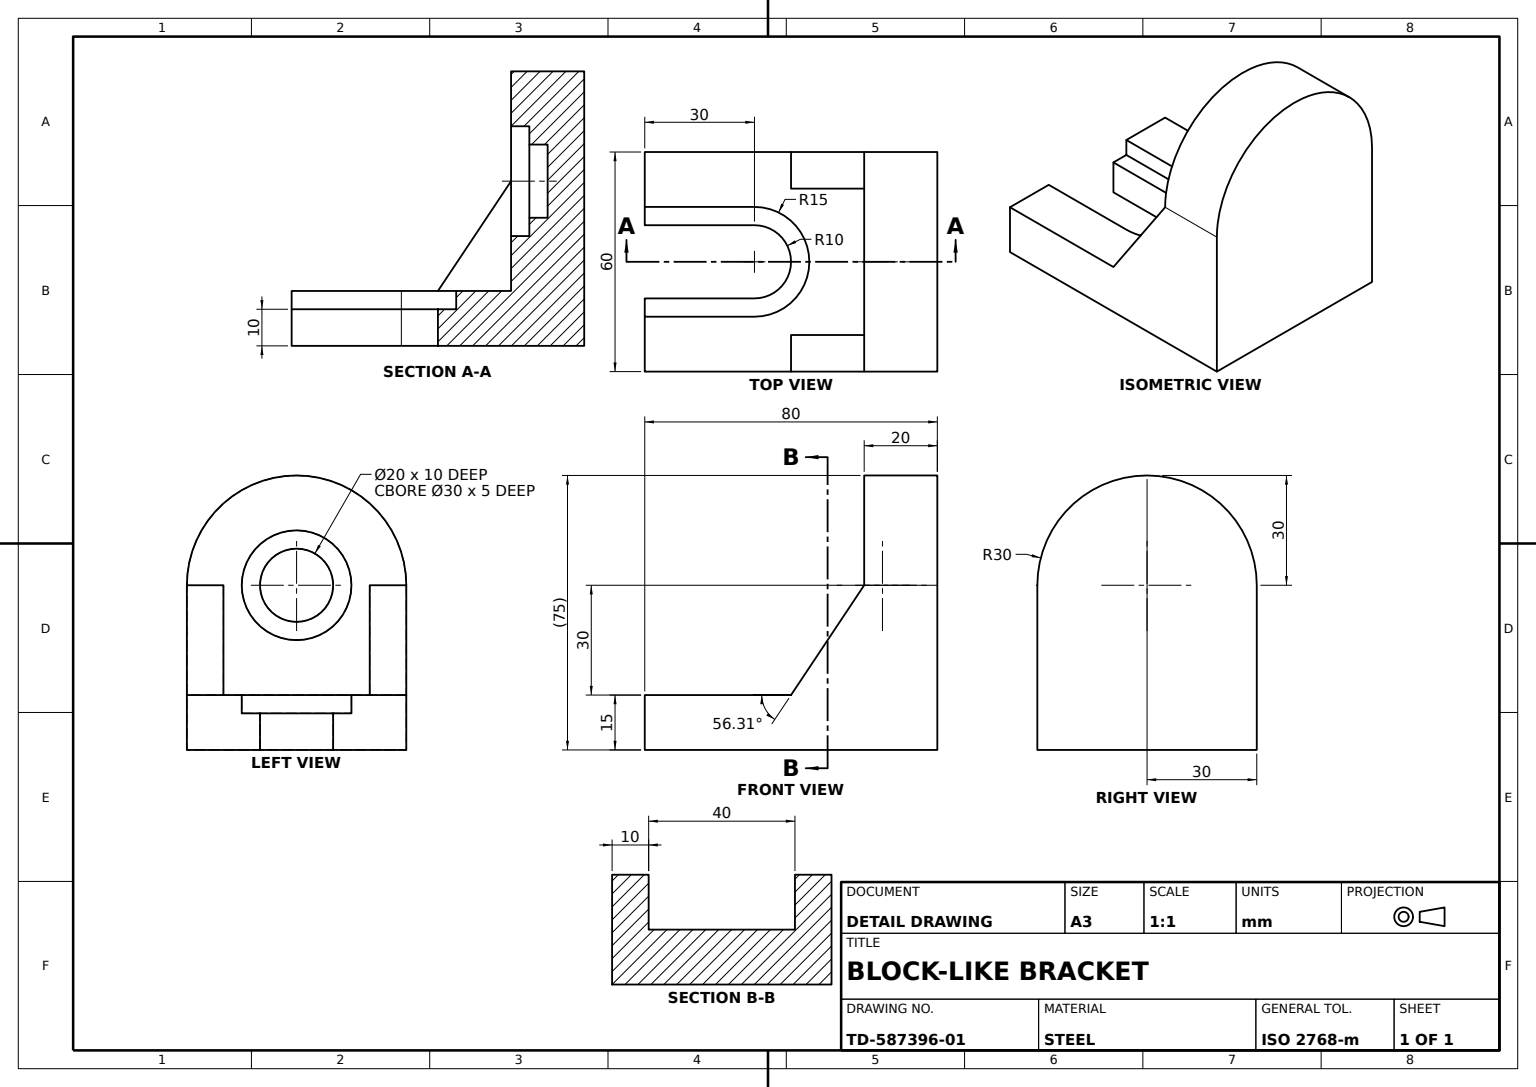
SolidWorks part; units mm, degrees
material "Plain Carbon Steel"
ref_plane "Front Plane" through (0, 0, 0) normal (0, 0, 1) x (1, 0, 0)
ref_plane "Top Plane" through (0, 0, 0) normal (0, 1, 0) x (1, 0, 0)
ref_plane "Right Plane" through (0, 0, 0) normal (1, 0, 0) x (0, 0, -1)
sketch "Base Plate Sketch" plane through (0, 0, 0) normal (0, 0, 1) x (1, 0, 0)
  line L0 (0, 0) -> (80, 0)
  line L1 (80, 0) -> (80, 60)
  line L2 (80, 60) -> (0, 60)
  line L3 (0, 60) -> (0, 0)
  dimension "D1" = 80
  dimension "D2" = 60
extrude "Base Plate" add sketch "Base Plate Sketch" along normal blind 15
sketch "Upright Block Sketch" plane through (80, 0, 0) normal (1, 0, 0) x (0, 0, -1)
  line L0 (-15, 60) -> (-45, 60)
  line L2 (-45, 0) -> (-15, 0)
  line L3 (-15, 0) -> (-15, 60) construction
  line L4 (-15, 0) -> (-15, 60)
  arc A0 (-45, 60) -> (-45, 0) centre (-45, 30) ccw
  dimension "D1" = 60
extrude "Upright Block" add sketch "Upright Block Sketch" against normal blind 20
sketch "Recess Ø30 Sketch" plane through (60, 0, 0) normal (-1, 0, 0) x (0, 0, 1)
  circle A0 centre (45, 30) radius 15
  dimension "D1" = 30
  dimension "D2" = 30
extrude "Recess Ø30" cut sketch "Recess Ø30 Sketch" against normal blind 5
sketch "Recess Ø20 Sketch" plane through (65, 0, 0) normal (-1, 0, 0) x (0, 0, 1)
  circle A0 centre (45, 30) radius 10
  dimension "D1" = 20
  dimension "D2" = 20
extrude "Recess Ø20" cut sketch "Recess Ø20 Sketch" against normal blind 5
sketch "Slot 30 Sketch" plane through (0, 0, 15) normal (0, 0, 1) x (1, 0, 0)
  line L0 (0, 45) -> (0, 15)
  line L1 (0, 60) -> (0, 0) construction
  line L2 (0, 45) -> (30, 45)
  line L4 (30, 15) -> (0, 15)
  line L5 (0, 0) -> (60, 0) construction
  arc A0 (30, 15) -> (30, 45) centre (30, 30) ccw
  dimension "D1" = 30
  dimension "D2" = 15
  dimension "D3" = 30
extrude "Slot 30" cut sketch "Slot 30 Sketch" against normal blind 5
sketch "Slot Step 20 Sketch" plane through (0, 0, 10) normal (0, 0, 1) x (1, 0, 0)
  line L0 (30, 45) -> (0, 45) construction
  line L1 (0, 45) -> (0, 15) construction
  line L2 (0, 40) -> (30, 40)
  line L4 (0, 20) -> (30, 20)
  line L5 (0, 40) -> (0, 20)
  arc A0 (30, 20) -> (30, 40) centre (30, 30) ccw
  dimension "D1" = 20
  dimension "D2" = 10
  dimension "D3" = 30
  dimension "D4" = 15
extrude "Slot Step 20" cut sketch "Slot Step 20 Sketch" against normal blind 10
sketch "Side Boss Sketch" plane through (0, 0, 0) normal (0, -1, 0) x (1, 0, 0)
  line L0 (60, 45) -> (40, 15)
  line L1 (0, 15) -> (60, 15) construction
  line L2 (60, 45) -> (80, 45) construction
  line L3 (60, 45) -> (60, 15)
  line L4 (60, 15) -> (40, 15)
  point P7 (70, 45)
  dimension "D1" = 30
extrude "Side Boss" add sketch "Side Boss Sketch" against normal blind 10
sketch "Rounded Boss Sketch" plane through (0, 60, 0) normal (0, 1, 0) x (1, 0, 0)
  line L0 (40, -15) -> (60, -15)
  line L1 (60, -15) -> (60, -45)
  line L2 (60, -45) -> (40, -15)
extrude "Rounded Boss" add sketch "Rounded Boss Sketch" against normal blind 10
